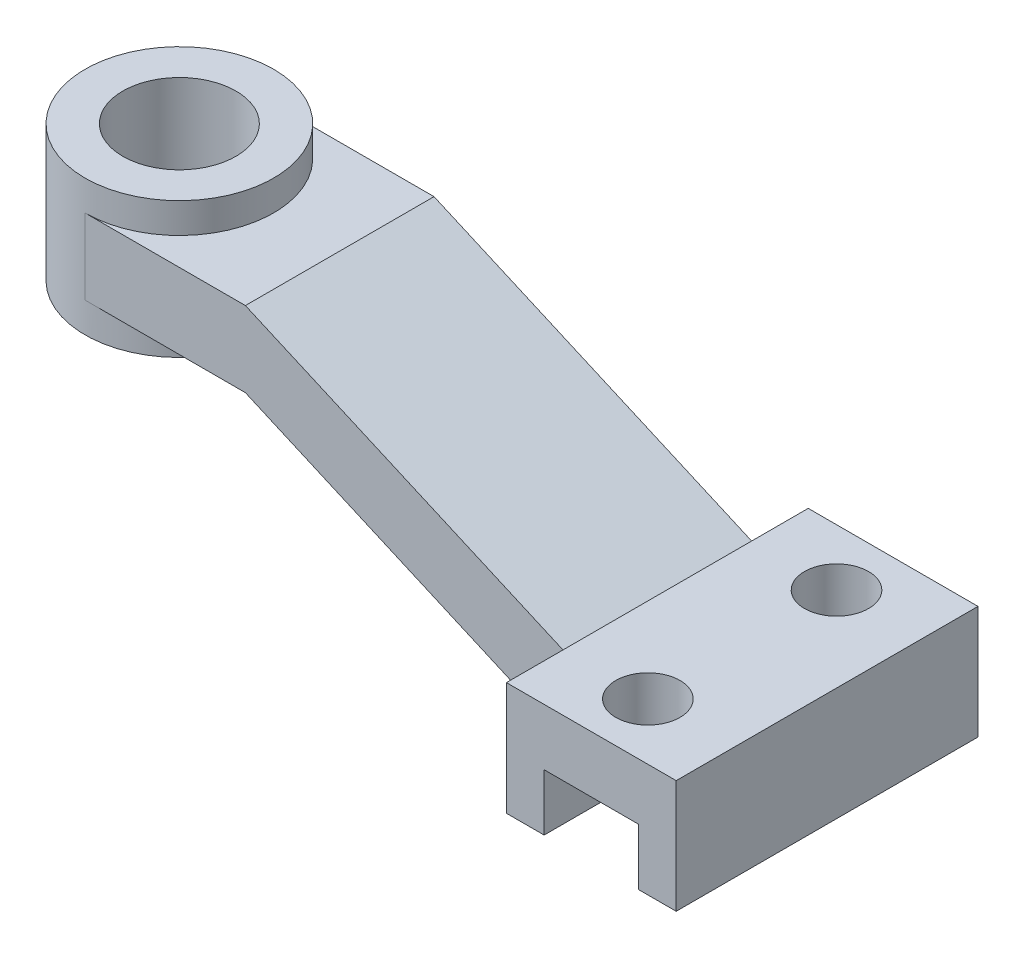
ISO-10303-21;
HEADER;
FILE_DESCRIPTION(('STEP AP214'),'2;1');
FILE_NAME('part.step','',(''),(''),'','','');
FILE_SCHEMA(('AUTOMOTIVE_DESIGN { 1 0 10303 214 1 1 1 1 }'));
ENDSEC;
DATA;
#1=APPLICATION_CONTEXT('core data for automotive mechanical design processes');
#2=APPLICATION_PROTOCOL_DEFINITION('international standard','automotive_design',2000,#1);
#3=PRODUCT_CONTEXT('',#1,'mechanical');
#4=PRODUCT('Part','Part','',(#3));
#5=PRODUCT_RELATED_PRODUCT_CATEGORY('part','',(#4));
#6=PRODUCT_DEFINITION_FORMATION('','',#4);
#7=PRODUCT_DEFINITION_CONTEXT('part definition',#1,'design');
#8=PRODUCT_DEFINITION('design','',#6,#7);
#9=PRODUCT_DEFINITION_SHAPE('','',#8);
#10=(LENGTH_UNIT() NAMED_UNIT(*) SI_UNIT(.MILLI.,.METRE.));
#11=(NAMED_UNIT(*) PLANE_ANGLE_UNIT() SI_UNIT($,.RADIAN.));
#12=(NAMED_UNIT(*) SI_UNIT($,.STERADIAN.) SOLID_ANGLE_UNIT());
#13=UNCERTAINTY_MEASURE_WITH_UNIT(LENGTH_MEASURE(1.E-05),#10,'distance_accuracy_value','');
#14=(GEOMETRIC_REPRESENTATION_CONTEXT(3) GLOBAL_UNCERTAINTY_ASSIGNED_CONTEXT((#13)) GLOBAL_UNIT_ASSIGNED_CONTEXT((#10,
#11,#12)) REPRESENTATION_CONTEXT('',''));
#15=CARTESIAN_POINT('',(0.,0.,0.));
#16=DIRECTION('',(0.,0.,1.));
#17=DIRECTION('',(1.,0.,0.));
#18=AXIS2_PLACEMENT_3D('',#15,#16,#17);
#19=CARTESIAN_POINT('',(0.,30.,80.));
#20=DIRECTION('',(1.,0.,0.));
#21=DIRECTION('',(0.,0.,-1.));
#22=AXIS2_PLACEMENT_3D('',#19,#20,#21);
#23=PLANE('',#22);
#24=DIRECTION('',(0.,0.,1.));
#25=VECTOR('',#24,1.);
#26=CARTESIAN_POINT('',(0.,10.,20.));
#27=LINE('',#26,#25);
#28=CARTESIAN_POINT('',(0.,10.,15.));
#29=VERTEX_POINT('',#28);
#30=CARTESIAN_POINT('',(0.,10.,65.));
#31=VERTEX_POINT('',#30);
#32=EDGE_CURVE('E160',#29,#31,#27,.T.);
#33=ORIENTED_EDGE('',*,*,#32,.F.);
#34=DIRECTION('',(0.,-1.,0.));
#35=VECTOR('',#34,1.);
#36=CARTESIAN_POINT('',(0.,10.,15.));
#37=LINE('',#36,#35);
#38=CARTESIAN_POINT('',(0.,30.,15.));
#39=VERTEX_POINT('',#38);
#40=EDGE_CURVE('E216',#39,#29,#37,.T.);
#41=ORIENTED_EDGE('',*,*,#40,.F.);
#42=DIRECTION('',(0.,0.,-1.));
#43=VECTOR('',#42,1.);
#44=CARTESIAN_POINT('',(0.,30.,80.));
#45=LINE('',#44,#43);
#46=CARTESIAN_POINT('',(0.,30.,0.));
#47=VERTEX_POINT('',#46);
#48=EDGE_CURVE('E101',#39,#47,#45,.T.);
#49=ORIENTED_EDGE('',*,*,#48,.T.);
#50=DIRECTION('',(0.,-1.,0.));
#51=VECTOR('',#50,1.);
#52=CARTESIAN_POINT('',(0.,30.,0.));
#53=LINE('',#52,#51);
#54=CARTESIAN_POINT('',(0.,0.,0.));
#55=VERTEX_POINT('',#54);
#56=EDGE_CURVE('E154',#47,#55,#53,.T.);
#57=ORIENTED_EDGE('',*,*,#56,.T.);
#58=DIRECTION('',(0.,0.,-1.));
#59=VECTOR('',#58,1.);
#60=CARTESIAN_POINT('',(0.,0.,80.));
#61=LINE('',#60,#59);
#62=CARTESIAN_POINT('',(0.,0.,80.));
#63=VERTEX_POINT('',#62);
#64=EDGE_CURVE('E11',#63,#55,#61,.T.);
#65=ORIENTED_EDGE('',*,*,#64,.F.);
#66=DIRECTION('',(0.,-1.,0.));
#67=VECTOR('',#66,1.);
#68=CARTESIAN_POINT('',(0.,30.,80.));
#69=LINE('',#68,#67);
#70=CARTESIAN_POINT('',(0.,30.,80.));
#71=VERTEX_POINT('',#70);
#72=EDGE_CURVE('E109',#71,#63,#69,.T.);
#73=ORIENTED_EDGE('',*,*,#72,.F.);
#74=CARTESIAN_POINT('',(0.,30.,65.));
#75=VERTEX_POINT('',#74);
#76=EDGE_CURVE('E167',#71,#75,#45,.T.);
#77=ORIENTED_EDGE('',*,*,#76,.T.);
#78=DIRECTION('',(0.,1.,0.));
#79=VECTOR('',#78,1.);
#80=CARTESIAN_POINT('',(0.,30.,65.));
#81=LINE('',#80,#79);
#82=EDGE_CURVE('E210',#31,#75,#81,.T.);
#83=ORIENTED_EDGE('',*,*,#82,.F.);
#84=EDGE_LOOP('',(#33,#41,#49,#57,#65,#73,#77,#83));
#85=FACE_BOUND('',#84,.T.);
#86=ADVANCED_FACE('F44',(#85),#23,.F.);
#87=CARTESIAN_POINT('',(0.,0.,80.));
#88=DIRECTION('',(0.,1.,0.));
#89=DIRECTION('',(0.,0.,1.));
#90=AXIS2_PLACEMENT_3D('',#87,#88,#89);
#91=PLANE('',#90);
#92=DIRECTION('',(1.,0.,0.));
#93=VECTOR('',#92,1.);
#94=CARTESIAN_POINT('',(0.,0.,0.));
#95=LINE('',#94,#93);
#96=CARTESIAN_POINT('',(10.,0.,0.));
#97=VERTEX_POINT('',#96);
#98=EDGE_CURVE('E156',#55,#97,#95,.T.);
#99=ORIENTED_EDGE('',*,*,#98,.T.);
#100=DIRECTION('',(0.,0.,-1.));
#101=VECTOR('',#100,1.);
#102=CARTESIAN_POINT('',(10.,0.,80.));
#103=LINE('',#102,#101);
#104=CARTESIAN_POINT('',(10.,0.,80.));
#105=VERTEX_POINT('',#104);
#106=EDGE_CURVE('E52',#105,#97,#103,.T.);
#107=ORIENTED_EDGE('',*,*,#106,.F.);
#108=DIRECTION('',(1.,0.,0.));
#109=VECTOR('',#108,1.);
#110=CARTESIAN_POINT('',(0.,0.,80.));
#111=LINE('',#110,#109);
#112=EDGE_CURVE('E200',#63,#105,#111,.T.);
#113=ORIENTED_EDGE('',*,*,#112,.F.);
#114=ORIENTED_EDGE('',*,*,#64,.T.);
#115=EDGE_LOOP('',(#99,#107,#113,#114));
#116=FACE_BOUND('',#115,.T.);
#117=ADVANCED_FACE('F305',(#116),#91,.F.);
#118=CARTESIAN_POINT('',(10.,0.,80.));
#119=DIRECTION('',(-1.,0.,0.));
#120=DIRECTION('',(0.,0.,1.));
#121=AXIS2_PLACEMENT_3D('',#118,#119,#120);
#122=PLANE('',#121);
#123=DIRECTION('',(0.,1.,0.));
#124=VECTOR('',#123,1.);
#125=CARTESIAN_POINT('',(10.,0.,0.));
#126=LINE('',#125,#124);
#127=CARTESIAN_POINT('',(10.,15.,0.));
#128=VERTEX_POINT('',#127);
#129=EDGE_CURVE('E157',#97,#128,#126,.T.);
#130=ORIENTED_EDGE('',*,*,#129,.T.);
#131=DIRECTION('',(0.,0.,-1.));
#132=VECTOR('',#131,1.);
#133=CARTESIAN_POINT('',(10.,15.,80.));
#134=LINE('',#133,#132);
#135=CARTESIAN_POINT('',(10.,15.,80.));
#136=VERTEX_POINT('',#135);
#137=EDGE_CURVE('E177',#136,#128,#134,.T.);
#138=ORIENTED_EDGE('',*,*,#137,.F.);
#139=DIRECTION('',(0.,1.,0.));
#140=VECTOR('',#139,1.);
#141=CARTESIAN_POINT('',(10.,0.,80.));
#142=LINE('',#141,#140);
#143=EDGE_CURVE('E186',#105,#136,#142,.T.);
#144=ORIENTED_EDGE('',*,*,#143,.F.);
#145=ORIENTED_EDGE('',*,*,#106,.T.);
#146=EDGE_LOOP('',(#130,#138,#144,#145));
#147=FACE_BOUND('',#146,.T.);
#148=ADVANCED_FACE('F190',(#147),#122,.F.);
#149=CARTESIAN_POINT('',(10.,15.,80.));
#150=DIRECTION('',(0.,1.,0.));
#151=DIRECTION('',(0.,0.,1.));
#152=AXIS2_PLACEMENT_3D('',#149,#150,#151);
#153=PLANE('',#152);
#154=CARTESIAN_POINT('',(22.5,15.,15.));
#155=DIRECTION('',(0.,1.,0.));
#156=DIRECTION('',(0.,0.,1.));
#157=AXIS2_PLACEMENT_3D('',#154,#155,#156);
#158=CIRCLE('',#157,8.5);
#159=CARTESIAN_POINT('',(22.5,15.,23.5));
#160=VERTEX_POINT('',#159);
#161=EDGE_CURVE('E221',#160,#160,#158,.T.);
#162=ORIENTED_EDGE('',*,*,#161,.T.);
#163=EDGE_LOOP('',(#162));
#164=FACE_BOUND('',#163,.T.);
#165=CARTESIAN_POINT('',(22.5,15.,65.));
#166=DIRECTION('',(0.,1.,0.));
#167=DIRECTION('',(0.,0.,1.));
#168=AXIS2_PLACEMENT_3D('',#165,#166,#167);
#169=CIRCLE('',#168,8.49999999999999);
#170=CARTESIAN_POINT('',(22.5,15.,73.5));
#171=VERTEX_POINT('',#170);
#172=EDGE_CURVE('E224',#171,#171,#169,.T.);
#173=ORIENTED_EDGE('',*,*,#172,.T.);
#174=EDGE_LOOP('',(#173));
#175=FACE_BOUND('',#174,.T.);
#176=DIRECTION('',(1.,0.,0.));
#177=VECTOR('',#176,1.);
#178=CARTESIAN_POINT('',(10.,15.,0.));
#179=LINE('',#178,#177);
#180=CARTESIAN_POINT('',(35.,15.,0.));
#181=VERTEX_POINT('',#180);
#182=EDGE_CURVE('E163',#128,#181,#179,.T.);
#183=ORIENTED_EDGE('',*,*,#182,.T.);
#184=DIRECTION('',(0.,0.,-1.));
#185=VECTOR('',#184,1.);
#186=CARTESIAN_POINT('',(35.,15.,80.));
#187=LINE('',#186,#185);
#188=CARTESIAN_POINT('',(35.,15.,80.));
#189=VERTEX_POINT('',#188);
#190=EDGE_CURVE('E141',#189,#181,#187,.T.);
#191=ORIENTED_EDGE('',*,*,#190,.F.);
#192=DIRECTION('',(1.,0.,0.));
#193=VECTOR('',#192,1.);
#194=CARTESIAN_POINT('',(10.,15.,80.));
#195=LINE('',#194,#193);
#196=EDGE_CURVE('E133',#136,#189,#195,.T.);
#197=ORIENTED_EDGE('',*,*,#196,.F.);
#198=ORIENTED_EDGE('',*,*,#137,.T.);
#199=EDGE_LOOP('',(#183,#191,#197,#198));
#200=FACE_BOUND('',#199,.T.);
#201=ADVANCED_FACE('F198',(#164,#175,#200),#153,.F.);
#202=CARTESIAN_POINT('',(35.,15.,80.));
#203=DIRECTION('',(1.,0.,0.));
#204=DIRECTION('',(0.,0.,-1.));
#205=AXIS2_PLACEMENT_3D('',#202,#203,#204);
#206=PLANE('',#205);
#207=DIRECTION('',(0.,-1.,0.));
#208=VECTOR('',#207,1.);
#209=CARTESIAN_POINT('',(35.,15.,0.));
#210=LINE('',#209,#208);
#211=CARTESIAN_POINT('',(35.,0.,0.));
#212=VERTEX_POINT('',#211);
#213=EDGE_CURVE('E139',#181,#212,#210,.T.);
#214=ORIENTED_EDGE('',*,*,#213,.T.);
#215=DIRECTION('',(0.,0.,-1.));
#216=VECTOR('',#215,1.);
#217=CARTESIAN_POINT('',(35.,0.,80.));
#218=LINE('',#217,#216);
#219=CARTESIAN_POINT('',(35.,0.,80.));
#220=VERTEX_POINT('',#219);
#221=EDGE_CURVE('E140',#220,#212,#218,.T.);
#222=ORIENTED_EDGE('',*,*,#221,.F.);
#223=DIRECTION('',(0.,-1.,0.));
#224=VECTOR('',#223,1.);
#225=CARTESIAN_POINT('',(35.,15.,80.));
#226=LINE('',#225,#224);
#227=EDGE_CURVE('E121',#189,#220,#226,.T.);
#228=ORIENTED_EDGE('',*,*,#227,.F.);
#229=ORIENTED_EDGE('',*,*,#190,.T.);
#230=EDGE_LOOP('',(#214,#222,#228,#229));
#231=FACE_BOUND('',#230,.T.);
#232=ADVANCED_FACE('F138',(#231),#206,.F.);
#233=CARTESIAN_POINT('',(35.,0.,80.));
#234=DIRECTION('',(0.,1.,0.));
#235=DIRECTION('',(0.,0.,1.));
#236=AXIS2_PLACEMENT_3D('',#233,#234,#235);
#237=PLANE('',#236);
#238=DIRECTION('',(1.,0.,0.));
#239=VECTOR('',#238,1.);
#240=CARTESIAN_POINT('',(35.,0.,0.));
#241=LINE('',#240,#239);
#242=CARTESIAN_POINT('',(45.,0.,0.));
#243=VERTEX_POINT('',#242);
#244=EDGE_CURVE('E165',#212,#243,#241,.T.);
#245=ORIENTED_EDGE('',*,*,#244,.T.);
#246=DIRECTION('',(0.,0.,-1.));
#247=VECTOR('',#246,1.);
#248=CARTESIAN_POINT('',(45.,0.,80.));
#249=LINE('',#248,#247);
#250=CARTESIAN_POINT('',(45.,0.,80.));
#251=VERTEX_POINT('',#250);
#252=EDGE_CURVE('E144',#251,#243,#249,.T.);
#253=ORIENTED_EDGE('',*,*,#252,.F.);
#254=DIRECTION('',(1.,0.,0.));
#255=VECTOR('',#254,1.);
#256=CARTESIAN_POINT('',(35.,0.,80.));
#257=LINE('',#256,#255);
#258=EDGE_CURVE('E130',#220,#251,#257,.T.);
#259=ORIENTED_EDGE('',*,*,#258,.F.);
#260=ORIENTED_EDGE('',*,*,#221,.T.);
#261=EDGE_LOOP('',(#245,#253,#259,#260));
#262=FACE_BOUND('',#261,.T.);
#263=ADVANCED_FACE('F149',(#262),#237,.F.);
#264=CARTESIAN_POINT('',(45.,0.,80.));
#265=DIRECTION('',(-1.,0.,0.));
#266=DIRECTION('',(0.,0.,1.));
#267=AXIS2_PLACEMENT_3D('',#264,#265,#266);
#268=PLANE('',#267);
#269=DIRECTION('',(0.,1.,0.));
#270=VECTOR('',#269,1.);
#271=CARTESIAN_POINT('',(45.,0.,0.));
#272=LINE('',#271,#270);
#273=CARTESIAN_POINT('',(45.,30.,0.));
#274=VERTEX_POINT('',#273);
#275=EDGE_CURVE('E168',#243,#274,#272,.T.);
#276=ORIENTED_EDGE('',*,*,#275,.T.);
#277=DIRECTION('',(0.,0.,-1.));
#278=VECTOR('',#277,1.);
#279=CARTESIAN_POINT('',(45.,30.,80.));
#280=LINE('',#279,#278);
#281=CARTESIAN_POINT('',(45.,30.,80.));
#282=VERTEX_POINT('',#281);
#283=EDGE_CURVE('E173',#282,#274,#280,.T.);
#284=ORIENTED_EDGE('',*,*,#283,.F.);
#285=DIRECTION('',(0.,1.,0.));
#286=VECTOR('',#285,1.);
#287=CARTESIAN_POINT('',(45.,0.,80.));
#288=LINE('',#287,#286);
#289=EDGE_CURVE('E69',#251,#282,#288,.T.);
#290=ORIENTED_EDGE('',*,*,#289,.F.);
#291=ORIENTED_EDGE('',*,*,#252,.T.);
#292=EDGE_LOOP('',(#276,#284,#290,#291));
#293=FACE_BOUND('',#292,.T.);
#294=ADVANCED_FACE('F385',(#293),#268,.F.);
#295=CARTESIAN_POINT('',(45.,30.,80.));
#296=DIRECTION('',(0.,-1.,0.));
#297=DIRECTION('',(0.,0.,-1.));
#298=AXIS2_PLACEMENT_3D('',#295,#296,#297);
#299=PLANE('',#298);
#300=CARTESIAN_POINT('',(22.5,30.,15.));
#301=DIRECTION('',(0.,1.,0.));
#302=DIRECTION('',(0.,0.,1.));
#303=AXIS2_PLACEMENT_3D('',#300,#301,#302);
#304=CIRCLE('',#303,8.5);
#305=CARTESIAN_POINT('',(22.5,30.,23.5));
#306=VERTEX_POINT('',#305);
#307=EDGE_CURVE('E230',#306,#306,#304,.T.);
#308=ORIENTED_EDGE('',*,*,#307,.F.);
#309=EDGE_LOOP('',(#308));
#310=FACE_BOUND('',#309,.T.);
#311=CARTESIAN_POINT('',(22.5,30.,65.));
#312=DIRECTION('',(0.,1.,0.));
#313=DIRECTION('',(0.,0.,1.));
#314=AXIS2_PLACEMENT_3D('',#311,#312,#313);
#315=CIRCLE('',#314,8.49999999999999);
#316=CARTESIAN_POINT('',(22.5,30.,73.5));
#317=VERTEX_POINT('',#316);
#318=EDGE_CURVE('E225',#317,#317,#315,.T.);
#319=ORIENTED_EDGE('',*,*,#318,.F.);
#320=EDGE_LOOP('',(#319));
#321=FACE_BOUND('',#320,.T.);
#322=DIRECTION('',(-1.,0.,0.));
#323=VECTOR('',#322,1.);
#324=CARTESIAN_POINT('',(45.,30.,0.));
#325=LINE('',#324,#323);
#326=EDGE_CURVE('E166',#274,#47,#325,.T.);
#327=ORIENTED_EDGE('',*,*,#326,.T.);
#328=ORIENTED_EDGE('',*,*,#48,.F.);
#329=EDGE_CURVE('E172',#75,#39,#45,.T.);
#330=ORIENTED_EDGE('',*,*,#329,.F.);
#331=ORIENTED_EDGE('',*,*,#76,.F.);
#332=DIRECTION('',(-1.,0.,0.));
#333=VECTOR('',#332,1.);
#334=CARTESIAN_POINT('',(45.,30.,80.));
#335=LINE('',#334,#333);
#336=EDGE_CURVE('E148',#282,#71,#335,.T.);
#337=ORIENTED_EDGE('',*,*,#336,.F.);
#338=ORIENTED_EDGE('',*,*,#283,.T.);
#339=EDGE_LOOP('',(#327,#328,#330,#331,#337,#338));
#340=FACE_BOUND('',#339,.T.);
#341=ADVANCED_FACE('F331',(#310,#321,#340),#299,.F.);
#342=CARTESIAN_POINT('',(0.,0.,80.));
#343=DIRECTION('',(0.,0.,1.));
#344=DIRECTION('',(1.,0.,0.));
#345=AXIS2_PLACEMENT_3D('',#342,#343,#344);
#346=PLANE('',#345);
#347=ORIENTED_EDGE('',*,*,#336,.T.);
#348=ORIENTED_EDGE('',*,*,#72,.T.);
#349=ORIENTED_EDGE('',*,*,#112,.T.);
#350=ORIENTED_EDGE('',*,*,#143,.T.);
#351=ORIENTED_EDGE('',*,*,#196,.T.);
#352=ORIENTED_EDGE('',*,*,#227,.T.);
#353=ORIENTED_EDGE('',*,*,#258,.T.);
#354=ORIENTED_EDGE('',*,*,#289,.T.);
#355=EDGE_LOOP('',(#347,#348,#349,#350,#351,#352,#353,#354));
#356=FACE_BOUND('',#355,.T.);
#357=ADVANCED_FACE('F129',(#356),#346,.T.);
#358=CARTESIAN_POINT('',(0.,0.,0.));
#359=DIRECTION('',(0.,0.,1.));
#360=DIRECTION('',(1.,0.,0.));
#361=AXIS2_PLACEMENT_3D('',#358,#359,#360);
#362=PLANE('',#361);
#363=ORIENTED_EDGE('',*,*,#56,.F.);
#364=ORIENTED_EDGE('',*,*,#326,.F.);
#365=ORIENTED_EDGE('',*,*,#275,.F.);
#366=ORIENTED_EDGE('',*,*,#244,.F.);
#367=ORIENTED_EDGE('',*,*,#213,.F.);
#368=ORIENTED_EDGE('',*,*,#182,.F.);
#369=ORIENTED_EDGE('',*,*,#129,.F.);
#370=ORIENTED_EDGE('',*,*,#98,.F.);
#371=EDGE_LOOP('',(#363,#364,#365,#366,#367,#368,#369,#370));
#372=FACE_BOUND('',#371,.T.);
#373=ADVANCED_FACE('F193',(#372),#362,.F.);
#374=CARTESIAN_POINT('',(-102.5,75.,20.));
#375=DIRECTION('',(0.401990062035198,0.915644030191284,0.));
#376=DIRECTION('',(-0.915644030191284,0.401990062035198,0.));
#377=AXIS2_PLACEMENT_3D('',#374,#375,#376);
#378=PLANE('',#377);
#379=DIRECTION('',(0.,0.,1.));
#380=VECTOR('',#379,1.);
#381=CARTESIAN_POINT('',(-84.1871193961743,66.960198759296,10.));
#382=LINE('',#381,#380);
#383=CARTESIAN_POINT('',(-84.1871193961743,66.960198759296,15.));
#384=VERTEX_POINT('',#383);
#385=CARTESIAN_POINT('',(-84.1871193961743,66.960198759296,65.));
#386=VERTEX_POINT('',#385);
#387=EDGE_CURVE('E228',#384,#386,#382,.T.);
#388=ORIENTED_EDGE('',*,*,#387,.T.);
#389=DIRECTION('',(-0.915644030191284,0.401990062035198,0.));
#390=VECTOR('',#389,1.);
#391=CARTESIAN_POINT('',(-102.5,75.,65.));
#392=LINE('',#391,#390);
#393=EDGE_CURVE('E202',#75,#386,#392,.T.);
#394=ORIENTED_EDGE('',*,*,#393,.F.);
#395=ORIENTED_EDGE('',*,*,#329,.T.);
#396=DIRECTION('',(0.915644030191284,-0.401990062035198,0.));
#397=VECTOR('',#396,1.);
#398=CARTESIAN_POINT('',(0.,30.,15.));
#399=LINE('',#398,#397);
#400=EDGE_CURVE('E215',#384,#39,#399,.T.);
#401=ORIENTED_EDGE('',*,*,#400,.F.);
#402=EDGE_LOOP('',(#388,#394,#395,#401));
#403=FACE_BOUND('',#402,.T.);
#404=ADVANCED_FACE('F326',(#403),#378,.T.);
#405=CARTESIAN_POINT('',(0.,10.,20.));
#406=DIRECTION('',(-0.401990062035198,-0.915644030191284,0.));
#407=DIRECTION('',(0.915644030191284,-0.401990062035198,0.));
#408=AXIS2_PLACEMENT_3D('',#405,#406,#407);
#409=PLANE('',#408);
#410=DIRECTION('',(0.,0.,1.));
#411=VECTOR('',#410,1.);
#412=CARTESIAN_POINT('',(-84.1871193961743,46.960198759296,10.));
#413=LINE('',#412,#411);
#414=CARTESIAN_POINT('',(-84.1871193961743,46.960198759296,15.));
#415=VERTEX_POINT('',#414);
#416=CARTESIAN_POINT('',(-84.1871193961743,46.960198759296,65.));
#417=VERTEX_POINT('',#416);
#418=EDGE_CURVE('E234',#415,#417,#413,.T.);
#419=ORIENTED_EDGE('',*,*,#418,.F.);
#420=DIRECTION('',(-0.915644030191284,0.401990062035198,0.));
#421=VECTOR('',#420,1.);
#422=CARTESIAN_POINT('',(-102.5,55.,15.));
#423=LINE('',#422,#421);
#424=EDGE_CURVE('E212',#29,#415,#423,.T.);
#425=ORIENTED_EDGE('',*,*,#424,.F.);
#426=ORIENTED_EDGE('',*,*,#32,.T.);
#427=DIRECTION('',(0.915644030191284,-0.401990062035198,0.));
#428=VECTOR('',#427,1.);
#429=CARTESIAN_POINT('',(0.,10.,65.));
#430=LINE('',#429,#428);
#431=EDGE_CURVE('E208',#417,#31,#430,.T.);
#432=ORIENTED_EDGE('',*,*,#431,.F.);
#433=EDGE_LOOP('',(#419,#425,#426,#432));
#434=FACE_BOUND('',#433,.T.);
#435=ADVANCED_FACE('F316',(#434),#409,.T.);
#436=CARTESIAN_POINT('',(0.,0.,65.));
#437=DIRECTION('',(0.,0.,-1.));
#438=DIRECTION('',(-1.,0.,0.));
#439=AXIS2_PLACEMENT_3D('',#436,#437,#438);
#440=PLANE('',#439);
#441=ORIENTED_EDGE('',*,*,#393,.T.);
#442=DIRECTION('',(-1.,0.,0.));
#443=VECTOR('',#442,1.);
#444=CARTESIAN_POINT('',(-84.1871193961743,66.960198759296,65.));
#445=LINE('',#444,#443);
#446=CARTESIAN_POINT('',(-126.687119396174,66.960198759296,65.));
#447=VERTEX_POINT('',#446);
#448=EDGE_CURVE('E246',#386,#447,#445,.T.);
#449=ORIENTED_EDGE('',*,*,#448,.T.);
#450=DIRECTION('',(0.,-1.,0.));
#451=VECTOR('',#450,1.);
#452=CARTESIAN_POINT('',(-126.687119396174,66.960198759296,65.));
#453=LINE('',#452,#451);
#454=CARTESIAN_POINT('',(-126.687119396174,46.960198759296,65.));
#455=VERTEX_POINT('',#454);
#456=EDGE_CURVE('E243',#447,#455,#453,.T.);
#457=ORIENTED_EDGE('',*,*,#456,.T.);
#458=DIRECTION('',(1.,0.,0.));
#459=VECTOR('',#458,1.);
#460=CARTESIAN_POINT('',(-126.687119396174,46.960198759296,65.));
#461=LINE('',#460,#459);
#462=EDGE_CURVE('E239',#455,#417,#461,.T.);
#463=ORIENTED_EDGE('',*,*,#462,.T.);
#464=ORIENTED_EDGE('',*,*,#431,.T.);
#465=ORIENTED_EDGE('',*,*,#82,.T.);
#466=EDGE_LOOP('',(#441,#449,#457,#463,#464,#465));
#467=FACE_BOUND('',#466,.T.);
#468=ADVANCED_FACE('F334',(#467),#440,.F.);
#469=CARTESIAN_POINT('',(0.,0.,15.));
#470=DIRECTION('',(0.,0.,1.));
#471=DIRECTION('',(1.,0.,0.));
#472=AXIS2_PLACEMENT_3D('',#469,#470,#471);
#473=PLANE('',#472);
#474=ORIENTED_EDGE('',*,*,#424,.T.);
#475=DIRECTION('',(1.,0.,0.));
#476=VECTOR('',#475,1.);
#477=CARTESIAN_POINT('',(-126.687119396174,46.960198759296,15.));
#478=LINE('',#477,#476);
#479=CARTESIAN_POINT('',(-126.687119396174,46.960198759296,15.));
#480=VERTEX_POINT('',#479);
#481=EDGE_CURVE('E240',#480,#415,#478,.T.);
#482=ORIENTED_EDGE('',*,*,#481,.F.);
#483=DIRECTION('',(0.,-1.,0.));
#484=VECTOR('',#483,1.);
#485=CARTESIAN_POINT('',(-126.687119396174,66.960198759296,15.));
#486=LINE('',#485,#484);
#487=CARTESIAN_POINT('',(-126.687119396174,66.960198759296,15.));
#488=VERTEX_POINT('',#487);
#489=EDGE_CURVE('E255',#488,#480,#486,.T.);
#490=ORIENTED_EDGE('',*,*,#489,.F.);
#491=DIRECTION('',(-1.,0.,0.));
#492=VECTOR('',#491,1.);
#493=CARTESIAN_POINT('',(-84.1871193961743,66.960198759296,15.));
#494=LINE('',#493,#492);
#495=EDGE_CURVE('E58',#384,#488,#494,.T.);
#496=ORIENTED_EDGE('',*,*,#495,.F.);
#497=ORIENTED_EDGE('',*,*,#400,.T.);
#498=ORIENTED_EDGE('',*,*,#40,.T.);
#499=EDGE_LOOP('',(#474,#482,#490,#496,#497,#498));
#500=FACE_BOUND('',#499,.T.);
#501=ADVANCED_FACE('F324',(#500),#473,.F.);
#502=CARTESIAN_POINT('',(22.5,15.,65.));
#503=DIRECTION('',(0.,1.,0.));
#504=DIRECTION('',(0.,0.,1.));
#505=AXIS2_PLACEMENT_3D('',#502,#503,#504);
#506=CYLINDRICAL_SURFACE('',#505,8.49999999999999);
#507=ORIENTED_EDGE('',*,*,#172,.F.);
#508=EDGE_LOOP('',(#507));
#509=FACE_BOUND('',#508,.T.);
#510=ORIENTED_EDGE('',*,*,#318,.T.);
#511=EDGE_LOOP('',(#510));
#512=FACE_BOUND('',#511,.T.);
#513=ADVANCED_FACE('F363',(#509,#512),#506,.F.);
#514=CARTESIAN_POINT('',(22.5,15.,15.));
#515=DIRECTION('',(0.,1.,0.));
#516=DIRECTION('',(0.,0.,1.));
#517=AXIS2_PLACEMENT_3D('',#514,#515,#516);
#518=CYLINDRICAL_SURFACE('',#517,8.5);
#519=ORIENTED_EDGE('',*,*,#161,.F.);
#520=EDGE_LOOP('',(#519));
#521=FACE_BOUND('',#520,.T.);
#522=ORIENTED_EDGE('',*,*,#307,.T.);
#523=EDGE_LOOP('',(#522));
#524=FACE_BOUND('',#523,.T.);
#525=ADVANCED_FACE('F357',(#521,#524),#518,.F.);
#526=CARTESIAN_POINT('',(-126.687119396174,46.960198759296,15.));
#527=DIRECTION('',(0.,-1.,0.));
#528=DIRECTION('',(0.,0.,-1.));
#529=AXIS2_PLACEMENT_3D('',#526,#527,#528);
#530=PLANE('',#529);
#531=ORIENTED_EDGE('',*,*,#462,.F.);
#532=CARTESIAN_POINT('',(-126.687119396174,46.960198759296,40.));
#533=DIRECTION('',(0.,-1.,0.));
#534=DIRECTION('',(0.,0.,-1.));
#535=AXIS2_PLACEMENT_3D('',#532,#533,#534);
#536=CIRCLE('',#535,25.);
#537=EDGE_CURVE('E265',#480,#455,#536,.T.);
#538=ORIENTED_EDGE('',*,*,#537,.F.);
#539=ORIENTED_EDGE('',*,*,#481,.T.);
#540=ORIENTED_EDGE('',*,*,#418,.T.);
#541=EDGE_LOOP('',(#531,#538,#539,#540));
#542=FACE_BOUND('',#541,.T.);
#543=ADVANCED_FACE('F294',(#542),#530,.T.);
#544=CARTESIAN_POINT('',(-84.1871193961743,66.960198759296,15.));
#545=DIRECTION('',(0.,1.,0.));
#546=DIRECTION('',(0.,0.,1.));
#547=AXIS2_PLACEMENT_3D('',#544,#545,#546);
#548=PLANE('',#547);
#549=CARTESIAN_POINT('',(-126.687119396174,66.960198759296,40.));
#550=DIRECTION('',(0.,1.,0.));
#551=DIRECTION('',(0.,0.,1.));
#552=AXIS2_PLACEMENT_3D('',#549,#550,#551);
#553=CIRCLE('',#552,25.);
#554=EDGE_CURVE('E259',#447,#488,#553,.T.);
#555=ORIENTED_EDGE('',*,*,#554,.F.);
#556=ORIENTED_EDGE('',*,*,#448,.F.);
#557=ORIENTED_EDGE('',*,*,#387,.F.);
#558=ORIENTED_EDGE('',*,*,#495,.T.);
#559=EDGE_LOOP('',(#555,#556,#557,#558));
#560=FACE_BOUND('',#559,.T.);
#561=ADVANCED_FACE('F282',(#560),#548,.T.);
#562=CARTESIAN_POINT('',(-126.687119396174,74.960198759296,40.));
#563=DIRECTION('',(0.,-1.,0.));
#564=DIRECTION('',(0.,0.,-1.));
#565=AXIS2_PLACEMENT_3D('',#562,#563,#564);
#566=CYLINDRICAL_SURFACE('',#565,25.);
#567=CARTESIAN_POINT('',(-126.687119396174,74.960198759296,40.));
#568=DIRECTION('',(0.,1.,0.));
#569=DIRECTION('',(0.,0.,1.));
#570=AXIS2_PLACEMENT_3D('',#567,#568,#569);
#571=CIRCLE('',#570,25.);
#572=CARTESIAN_POINT('',(-126.687119396174,74.960198759296,65.));
#573=VERTEX_POINT('',#572);
#574=EDGE_CURVE('E248',#573,#573,#571,.T.);
#575=ORIENTED_EDGE('',*,*,#574,.F.);
#576=EDGE_LOOP('',(#575));
#577=FACE_BOUND('',#576,.T.);
#578=ORIENTED_EDGE('',*,*,#554,.T.);
#579=ORIENTED_EDGE('',*,*,#489,.T.);
#580=ORIENTED_EDGE('',*,*,#537,.T.);
#581=ORIENTED_EDGE('',*,*,#456,.F.);
#582=EDGE_LOOP('',(#578,#579,#580,#581));
#583=FACE_BOUND('',#582,.T.);
#584=CARTESIAN_POINT('',(-126.687119396174,38.960198759296,40.));
#585=DIRECTION('',(0.,-1.,0.));
#586=DIRECTION('',(0.,0.,-1.));
#587=AXIS2_PLACEMENT_3D('',#584,#585,#586);
#588=CIRCLE('',#587,25.);
#589=CARTESIAN_POINT('',(-126.687119396174,38.960198759296,15.));
#590=VERTEX_POINT('',#589);
#591=EDGE_CURVE('E258',#590,#590,#588,.T.);
#592=ORIENTED_EDGE('',*,*,#591,.F.);
#593=EDGE_LOOP('',(#592));
#594=FACE_BOUND('',#593,.T.);
#595=ADVANCED_FACE('F281',(#577,#583,#594),#566,.T.);
#596=CARTESIAN_POINT('',(-126.687119396174,74.960198759296,40.));
#597=DIRECTION('',(0.,1.,0.));
#598=DIRECTION('',(0.,0.,1.));
#599=AXIS2_PLACEMENT_3D('',#596,#597,#598);
#600=PLANE('',#599);
#601=CARTESIAN_POINT('',(-126.687119396174,74.960198759296,40.));
#602=DIRECTION('',(0.,1.,0.));
#603=DIRECTION('',(0.,0.,1.));
#604=AXIS2_PLACEMENT_3D('',#601,#602,#603);
#605=CIRCLE('',#604,15.);
#606=CARTESIAN_POINT('',(-126.687119396174,74.960198759296,55.));
#607=VERTEX_POINT('',#606);
#608=EDGE_CURVE('E270',#607,#607,#605,.T.);
#609=ORIENTED_EDGE('',*,*,#608,.F.);
#610=EDGE_LOOP('',(#609));
#611=FACE_BOUND('',#610,.T.);
#612=ORIENTED_EDGE('',*,*,#574,.T.);
#613=EDGE_LOOP('',(#612));
#614=FACE_BOUND('',#613,.T.);
#615=ADVANCED_FACE('F278',(#611,#614),#600,.T.);
#616=CARTESIAN_POINT('',(-126.687119396174,38.960198759296,40.));
#617=DIRECTION('',(0.,-1.,0.));
#618=DIRECTION('',(0.,0.,-1.));
#619=AXIS2_PLACEMENT_3D('',#616,#617,#618);
#620=PLANE('',#619);
#621=CARTESIAN_POINT('',(-126.687119396174,38.960198759296,40.));
#622=DIRECTION('',(0.,-1.,0.));
#623=DIRECTION('',(0.,0.,-1.));
#624=AXIS2_PLACEMENT_3D('',#621,#622,#623);
#625=CIRCLE('',#624,15.);
#626=CARTESIAN_POINT('',(-126.687119396174,38.960198759296,25.));
#627=VERTEX_POINT('',#626);
#628=EDGE_CURVE('E48',#627,#627,#625,.T.);
#629=ORIENTED_EDGE('',*,*,#628,.F.);
#630=EDGE_LOOP('',(#629));
#631=FACE_BOUND('',#630,.T.);
#632=ORIENTED_EDGE('',*,*,#591,.T.);
#633=EDGE_LOOP('',(#632));
#634=FACE_BOUND('',#633,.T.);
#635=ADVANCED_FACE('F279',(#631,#634),#620,.T.);
#636=CARTESIAN_POINT('',(-126.687119396174,34.960198759296,40.));
#637=DIRECTION('',(0.,1.,0.));
#638=DIRECTION('',(0.,0.,1.));
#639=AXIS2_PLACEMENT_3D('',#636,#637,#638);
#640=CYLINDRICAL_SURFACE('',#639,15.);
#641=ORIENTED_EDGE('',*,*,#628,.T.);
#642=EDGE_LOOP('',(#641));
#643=FACE_BOUND('',#642,.T.);
#644=ORIENTED_EDGE('',*,*,#608,.T.);
#645=EDGE_LOOP('',(#644));
#646=FACE_BOUND('',#645,.T.);
#647=ADVANCED_FACE('F274',(#643,#646),#640,.F.);
#648=CLOSED_SHELL('',(#86,#117,#148,#201,#232,#263,#294,#341,#357,#373,#404,#435,#468,#501,#513,
#525,#543,#561,#595,#615,#635,#647));
#649=MANIFOLD_SOLID_BREP('B2',#648);
#650=ADVANCED_BREP_SHAPE_REPRESENTATION('',(#18,#649),#14);
#651=SHAPE_DEFINITION_REPRESENTATION(#9,#650);
ENDSEC;
END-ISO-10303-21;
